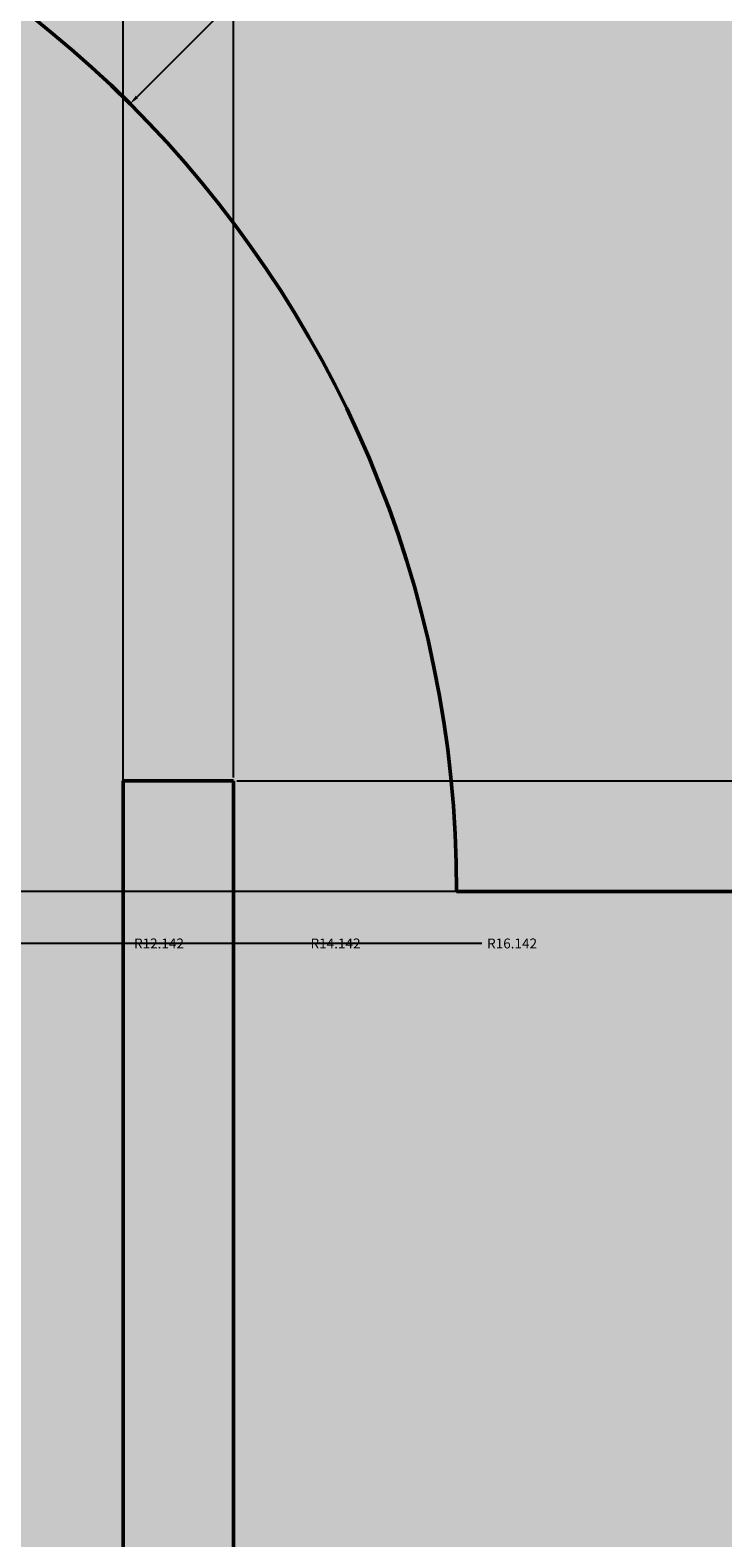
# Model space of a CAD drawing. Units: inches. Extents: x -12 to 334, y -10 to 186.
# Tile 55 of 77: x 244 to 257, y 69 to 96. Entities that reach past the tile are written whole.
import ezdxf

# ---------------------------------------------------------------- set-up
doc = ezdxf.new("R2010")
doc.units = ezdxf.units.IN
doc.header["$MEASUREMENT"] = 0
for name, color, linetype, lineweight in [('M-DIMS', 2, 'Continuous', 18), ('M-EQPM', 7, 'Continuous', 50), ('M-EQPM-PATT', 8, 'Continuous', 18)]:
    doc.layers.add(name, color=color, linetype=linetype, lineweight=lineweight)
doc.styles.get("Standard").update_dxf_attribs({"font": 'arial.ttf'})
doc.dimstyles.get("Standard").update_dxf_attribs({"dimtxt": 0.18, "dimasz": 0.18, "dimexe": 0.18, "dimexo": 0.0625, "dimgap": 0.09, "dimtad": 0, "dimtih": 1, "dimtoh": 1, "dimdec": 4, "dimzin": 0, "dimdsep": 46, "dimtxsty": 'Standard', "dimcen": 0.09, "dimadec": 0, "dimazin": 0, "dimtfac": 1, "dimtdec": 4, "dimtofl": 0, "dimtmove": 0, "dimatfit": 3, "dimfxl": 1, "dimtolj": 1, "dimtzin": 0, "dimarcsym": 0})

# ---------------------------------------------------------------- blocks, each defined once
blk = doc.blocks.new('*D1')
at = {"layer": 'Defpoints', "color": 0, "transparency": 16777216}
for p in [(281.426, 91.899), (3.376, 80.692), (281.426, 14.304)]:
    blk.add_point(p, dxfattribs=at)
at = {"layer": 'M-DIMS', "color": 0, "lineweight": -2, "transparency": 16777216}
for p, q in [((281.426, 91.836), (281.426, 14.124)), ((3.376, 80.629), (3.376, 14.124)), ((3.556, 14.304), (141.935, 14.304)), ((281.246, 14.304), (142.867, 14.304))]:
    blk.add_line(p, q, dxfattribs=at)
at = {"layer": 'M-DIMS', "color": 0, "transparency": 16777216}
for points in [[(3.556, 14.334), (3.556, 14.274), (3.376, 14.304)], [(281.246, 14.334), (281.246, 14.274), (281.426, 14.304)]]:
    blk.add_solid(points, dxfattribs=at)
at = {"layer": 'M-DIMS', "color": 0, "transparency": 16777216, "insert": (142.401, 14.304), "char_height": 0.18, "attachment_point": 5}
blk.add_mtext('\\A1;278.05', dxfattribs=at)
blk = doc.blocks.new('*D17')
at = {"layer": 'Defpoints', "color": 0, "transparency": 16777216}
for p in [(106.177, 102.896), (105.892, 56.321), (295.976, 56.321)]:
    blk.add_point(p, dxfattribs=at)
at = {"layer": 'M-DIMS', "color": 0, "lineweight": -2, "transparency": 16777216}
for p, q in [((106.24, 102.896), (296.156, 102.896)), ((295.976, 102.716), (295.976, 79.79)), ((295.976, 56.501), (295.976, 79.426)), ((105.954, 56.321), (296.156, 56.321))]:
    blk.add_line(p, q, dxfattribs=at)
at = {"layer": 'M-DIMS', "color": 0, "transparency": 16777216}
for points in [[(295.946, 102.716), (296.006, 102.716), (295.976, 102.896)], [(295.946, 56.501), (296.006, 56.501), (295.976, 56.321)]]:
    blk.add_solid(points, dxfattribs=at)
at = {"layer": 'M-DIMS', "color": 0, "transparency": 16777216, "insert": (295.976, 79.608), "char_height": 0.18, "attachment_point": 5}
blk.add_mtext('\\A1;46.575', dxfattribs=at)
blk = doc.blocks.new('*D36')
at = {"layer": 'Defpoints', "color": 0, "transparency": 16777216}
for p in [(247.935, 169.385), (245.935, 82.697), (247.935, 82.697)]:
    blk.add_point(p, dxfattribs=at)
at = {"layer": 'M-DIMS', "color": 0, "lineweight": -2, "transparency": 16777216}
for p, q in [((245.935, 82.759), (245.935, 169.565)), ((246.115, 169.385), (246.786, 169.385)), ((247.755, 169.385), (247.085, 169.385)), ((247.935, 82.759), (247.935, 169.565))]:
    blk.add_line(p, q, dxfattribs=at)
at = {"layer": 'M-DIMS', "color": 0, "transparency": 16777216}
for points in [[(246.115, 169.415), (246.115, 169.355), (245.935, 169.385)], [(247.755, 169.415), (247.755, 169.355), (247.935, 169.385)]]:
    blk.add_solid(points, dxfattribs=at)
at = {"layer": 'M-DIMS', "color": 0, "transparency": 16777216, "insert": (246.935, 169.385), "char_height": 0.18, "attachment_point": 5}
blk.add_mtext('\\A1;2', dxfattribs=at)
blk = doc.blocks.new('*D37')
at = {"layer": 'Defpoints', "color": 0, "transparency": 16777216}
for p in [(245.935, 169.385), (232.576, 46.854), (245.935, 46.854)]:
    blk.add_point(p, dxfattribs=at)
at = {"layer": 'M-DIMS', "color": 0, "lineweight": -2, "transparency": 16777216}
for p, q in [((232.576, 46.917), (232.576, 169.565)), ((232.756, 169.385), (238.871, 169.385)), ((245.755, 169.385), (239.641, 169.385)), ((245.935, 46.917), (245.935, 169.565))]:
    blk.add_line(p, q, dxfattribs=at)
at = {"layer": 'M-DIMS', "color": 0, "transparency": 16777216}
for points in [[(232.756, 169.415), (232.756, 169.355), (232.576, 169.385)], [(245.755, 169.415), (245.755, 169.355), (245.935, 169.385)]]:
    blk.add_solid(points, dxfattribs=at)
at = {"layer": 'M-DIMS', "color": 0, "transparency": 16777216, "insert": (239.256, 169.385), "char_height": 0.18, "attachment_point": 5}
blk.add_mtext('\\A1;13.36', dxfattribs=at)
blk = doc.blocks.new('*D38')
at = {"layer": 'Defpoints', "color": 0, "transparency": 16777216}
for p in [(247.935, 82.697), (247.935, 46.854), (295.976, 46.854)]:
    blk.add_point(p, dxfattribs=at)
at = {"layer": 'M-DIMS', "color": 0, "lineweight": -2, "transparency": 16777216}
for p, q in [((247.998, 82.697), (296.156, 82.697)), ((295.976, 82.517), (295.976, 64.957)), ((295.976, 47.034), (295.976, 64.594)), ((247.998, 46.854), (296.156, 46.854))]:
    blk.add_line(p, q, dxfattribs=at)
at = {"layer": 'M-DIMS', "color": 0, "transparency": 16777216}
for points in [[(295.946, 82.517), (296.006, 82.517), (295.976, 82.697)], [(295.946, 47.034), (296.006, 47.034), (295.976, 46.854)]]:
    blk.add_solid(points, dxfattribs=at)
at = {"layer": 'M-DIMS', "color": 0, "transparency": 16777216, "insert": (295.976, 64.775), "char_height": 0.18, "attachment_point": 5}
blk.add_mtext('\\A1;35.84', dxfattribs=at)
blk = doc.blocks.new('*D39')
at = {"layer": 'Defpoints', "color": 0, "transparency": 16777216}
for p in [(279.726, 80.692), (-11.174, 45.854), (269.381, 45.854)]:
    blk.add_point(p, dxfattribs=at)
at = {"layer": 'M-DIMS', "color": 0, "lineweight": -2, "transparency": 16777216}
for p, q in [((279.664, 80.692), (-11.354, 80.692)), ((-11.174, 80.512), (-11.174, 63.455)), ((-11.174, 46.034), (-11.174, 63.091)), ((269.318, 45.854), (-11.354, 45.854))]:
    blk.add_line(p, q, dxfattribs=at)
at = {"layer": 'M-DIMS', "color": 0, "transparency": 16777216}
for points in [[(-11.204, 80.512), (-11.144, 80.512), (-11.174, 80.692)], [(-11.204, 46.034), (-11.144, 46.034), (-11.174, 45.854)]]:
    blk.add_solid(points, dxfattribs=at)
at = {"layer": 'M-DIMS', "color": 0, "transparency": 16777216, "insert": (-11.174, 63.273), "char_height": 0.18, "attachment_point": 5}
blk.add_mtext('\\A1;34.84', dxfattribs=at)
blk = doc.blocks.new('*D40')
at = {"layer": 'Defpoints', "color": 0, "transparency": 16777216}
for p in [(278.229, 116.208), (187.394, 91.899)]:
    blk.add_point(p, dxfattribs=at)
at = {"layer": 'M-DIMS', "color": 0, "lineweight": -2, "transparency": 16777216}
for p, q in [((332.73, 130.793), (278.403, 116.254)), ((187.394, 91.809), (187.394, 91.989)), ((187.304, 91.899), (187.484, 91.899))]:
    blk.add_line(p, q, dxfattribs=at)
at = {"layer": 'M-DIMS', "color": 0, "transparency": 16777216}
blk.add_solid([(278.395, 116.283), (278.411, 116.225), (278.229, 116.208)], dxfattribs=at)
at = {"layer": 'M-DIMS', "color": 0, "transparency": 16777216, "insert": (333.21, 130.793), "char_height": 0.18, "attachment_point": 5}
blk.add_mtext('\\A1;R94.03', dxfattribs=at)
blk = doc.blocks.new('*D41')
at = {"layer": 'Defpoints', "color": 0, "transparency": 16777216}
for p in [(190.169, 91.899), (277.343, 68.515)]:
    blk.add_point(p, dxfattribs=at)
at = {"layer": 'M-DIMS', "color": 0, "lineweight": -2, "transparency": 16777216}
for p, q in [((190.169, 91.809), (190.169, 91.989)), ((190.079, 91.899), (190.259, 91.899)), ((329.648, 54.485), (277.517, 68.469)), ((329.828, 54.485), (329.648, 54.485))]:
    blk.add_line(p, q, dxfattribs=at)
at = {"layer": 'M-DIMS', "color": 0, "transparency": 16777216}
blk.add_solid([(277.525, 68.498), (277.509, 68.44), (277.343, 68.515)], dxfattribs=at)
at = {"layer": 'M-DIMS', "color": 0, "transparency": 16777216, "insert": (330.307, 54.485), "char_height": 0.18, "attachment_point": 5}
blk.add_mtext('\\A1;R90.26', dxfattribs=at)
blk = doc.blocks.new('*D43')
at = {"layer": 'Defpoints', "color": 0, "transparency": 16777216}
for p in [(246.06, 94.98), (231.776, 80.692)]:
    blk.add_point(p, dxfattribs=at)
at = {"layer": 'M-DIMS', "color": 0, "lineweight": -2, "transparency": 16777216}
for p, q in [((254.631, 103.553), (246.187, 95.108)), ((254.811, 103.553), (254.631, 103.553)), ((231.686, 80.692), (231.866, 80.692)), ((231.776, 80.602), (231.776, 80.782))]:
    blk.add_line(p, q, dxfattribs=at)
at = {"layer": 'M-DIMS', "color": 0, "transparency": 16777216}
blk.add_solid([(246.166, 95.129), (246.209, 95.086), (246.06, 94.98)], dxfattribs=at)
at = {"layer": 'M-DIMS', "color": 0, "transparency": 16777216, "insert": (255.36, 103.553), "char_height": 0.18, "attachment_point": 5}
blk.add_mtext('\\A1;R20.204', dxfattribs=at)
blk = doc.blocks.new('*D45')
at = {"layer": 'Defpoints', "color": 0, "transparency": 16777216}
for p in [(226.608, 79.754), (242.751, 79.75)]:
    blk.add_point(p, dxfattribs=at)
at = {"layer": 'M-DIMS', "color": 0, "lineweight": -2, "transparency": 16777216}
for p, q in [((226.518, 79.754), (226.698, 79.754)), ((226.608, 79.664), (226.608, 79.844)), ((252.436, 79.748), (242.931, 79.75))]:
    blk.add_line(p, q, dxfattribs=at)
at = {"layer": 'M-DIMS', "color": 0, "transparency": 16777216}
blk.add_solid([(242.931, 79.78), (242.931, 79.72), (242.751, 79.75)], dxfattribs=at)
at = {"layer": 'M-DIMS', "color": 0, "transparency": 16777216, "insert": (252.985, 79.748), "char_height": 0.18, "attachment_point": 5}
blk.add_mtext('\\A1;R16.142', dxfattribs=at)
blk = doc.blocks.new('*D46')
at = {"layer": 'Defpoints', "color": 0, "transparency": 16777216}
for p in [(226.608, 79.754), (240.751, 79.75)]:
    blk.add_point(p, dxfattribs=at)
at = {"layer": 'M-DIMS', "color": 0, "lineweight": -2, "transparency": 16777216}
for p, q in [((226.518, 79.754), (226.698, 79.754)), ((226.608, 79.664), (226.608, 79.844)), ((249.236, 79.748), (240.931, 79.75))]:
    blk.add_line(p, q, dxfattribs=at)
at = {"layer": 'M-DIMS', "color": 0, "transparency": 16777216}
blk.add_solid([(240.931, 79.78), (240.931, 79.72), (240.751, 79.75)], dxfattribs=at)
at = {"layer": 'M-DIMS', "color": 0, "transparency": 16777216, "insert": (249.785, 79.748), "char_height": 0.18, "attachment_point": 5}
blk.add_mtext('\\A1;R14.142', dxfattribs=at)
blk = doc.blocks.new('*D47')
at = {"layer": 'Defpoints', "color": 0, "transparency": 16777216}
for p in [(226.608, 79.754), (238.751, 79.75)]:
    blk.add_point(p, dxfattribs=at)
at = {"layer": 'M-DIMS', "color": 0, "lineweight": -2, "transparency": 16777216}
for p, q in [((226.518, 79.754), (226.698, 79.754)), ((226.608, 79.664), (226.608, 79.844)), ((246.036, 79.748), (238.931, 79.75))]:
    blk.add_line(p, q, dxfattribs=at)
at = {"layer": 'M-DIMS', "color": 0, "transparency": 16777216}
blk.add_solid([(238.931, 79.78), (238.931, 79.72), (238.751, 79.75)], dxfattribs=at)
at = {"layer": 'M-DIMS', "color": 0, "transparency": 16777216, "insert": (246.585, 79.748), "char_height": 0.18, "attachment_point": 5}
blk.add_mtext('\\A1;R12.142', dxfattribs=at)

msp = doc.modelspace()

# ---------------------------------------------------------------- hatches: boundary and pattern name
at = {"layer": 'M-EQPM-PATT', "transparency": 33554556}
h = msp.add_hatch(color=256, dxfattribs=at)
h.set_gradient(color1=(248, 206, 179), color2=(248, 206, 179), tint=1)
h.paths.add_polyline_path([(179.7818, 136.8871), (126.9567, 136.8871), (106.1771, 100.8958), (171.5458, 100.8958)])
h.paths.add_polyline_path([(268.3808, 136.9435), (214.0166, 136.9435), (214.0166, 154.8345), (196.3421, 154.8345), (196.3421, 136.8871), (179.7818, 136.8871), (171.5458, 100.8958), (231.7758, 100.8958, -0.4142136), (251.9801, 80.6915), (279.7263, 80.6915, 0.1631825)])
at = {"layer": 'M-EQPM-PATT'}
h = msp.add_hatch(color=256, dxfattribs=at)
h.set_gradient(color1=(94, 103, 175), color2=(94, 103, 175), tint=1)
h.paths.add_polyline_path([(129.093, 89.8963), (86.8879, 89.8963), (86.8879, 69.6117), (129.093, 69.6117)], flags=17)
h.paths.add_polyline_path([(170.9079, 89.8963), (130.8573, 89.8963), (130.8573, 69.6117), (170.9079, 69.6117)], flags=17)
h.paths.add_polyline_path([(216.4278, 89.8963), (172.6722, 89.8963), (172.6722, 69.6117), (216.4278, 69.6117)], flags=17)
h.paths.add_polyline_path([(245.9354, 82.6969), (247.9354, 82.6969), (247.9354, 46.8541), (268.3808, 46.8541, 0.0998398), (279.7263, 80.6915), (251.9801, 80.6915, 0.4142136), (231.7758, 100.8958), (84.7229, 100.8958), (84.7229, 109.0583), (83.7229, 109.0583), (83.7229, 95.8963), (129.093, 95.8963), (129.093, 98.1081), (130.8573, 98.1081), (130.8573, 95.8963), (170.9079, 95.8963), (170.9079, 98.1081), (172.6722, 98.1081), (172.6722, 95.8963), (216.4278, 95.8963), (216.4278, 98.1081), (218.1922, 98.1081), (218.1922, 95.8963), (226.6083, 95.8963, -1), (226.6083, 63.6117), (218.1922, 63.6117), (218.1922, 61.1045), (216.4278, 61.1045), (216.4278, 63.6117), (172.6722, 63.6117), (172.6722, 61.1045), (170.9079, 61.1045), (170.9079, 63.6117), (130.8573, 63.6117), (130.8573, 61.1045), (129.093, 61.1045), (129.093, 63.6117), (87.8879, 63.6117), (87.8879, 56.3205), (105.8919, 56.3205), (105.8919, 28.8541), (115.8919, 28.8541), (115.8919, 46.8541), (222.5761, 46.8541), (222.5761, 30.8541), (232.5761, 30.8541), (232.5761, 46.8541), (245.9354, 46.8541)])
h.paths.add_polyline_path([(86.8879, 89.8963), (75.9244, 89.8963), (75.9244, 69.6117), (86.8879, 69.6117)])
h.paths.add_polyline_path([(83.7229, 109.0583), (75.9244, 109.0583), (75.9244, 95.8963), (83.7229, 95.8963)])
h.paths.add_polyline_path([(226.6083, 89.8963), (218.1922, 89.8963), (218.1922, 69.6117), (226.6083, 69.6117, 1)], flags=17)
h = msp.add_hatch(color=256, dxfattribs=at)
h.set_gradient(color1=(0, 0, 255), color2=(0, 0, 255), tint=1)
h.paths.add_polyline_path([(84.7229, 100.8958), (84.7229, 109.0583), (83.7229, 109.0583), (83.7229, 95.8963), (129.093, 95.8963), (129.093, 98.1081), (130.8573, 98.1081), (130.8573, 95.8963), (170.9079, 95.8963), (170.9079, 98.1081), (172.6722, 98.1081), (172.6722, 95.8963), (216.4278, 95.8963), (216.4278, 98.1081), (218.1922, 98.1081), (218.1922, 95.8963), (226.6083, 95.8963, -1), (226.6083, 63.6117), (218.1922, 63.6117), (218.1922, 61.1045), (216.4278, 61.1045), (216.4278, 63.6117), (172.6722, 63.6117), (172.6722, 61.1045), (170.9079, 61.1045), (170.9079, 63.6117), (130.8573, 63.6117), (130.8573, 61.1045), (129.093, 61.1045), (129.093, 63.6117), (87.8879, 63.6117), (87.8879, 56.3205), (105.8919, 56.3205), (105.8919, 28.8541), (115.8919, 28.8541), (115.8919, 46.8541), (222.5761, 46.8541), (222.5761, 30.8541), (232.5761, 30.8541), (232.5761, 46.8541), (245.9354, 46.8541), (245.9354, 82.6969), (247.9354, 82.6969), (247.9354, 46.8541), (268.3808, 46.8541, 0.0998398), (279.7263, 80.6915), (251.9801, 80.6915, 0.4142136), (231.7758, 100.8958)])
h = msp.add_hatch(color=256, dxfattribs=at)
h.set_gradient(color1=(241, 235, 31), color2=(244, 238, 81), tint=1)
h.paths.add_polyline_path([(245.9354, 46.8541), (247.9354, 46.8541), (247.9354, 82.6969), (245.9354, 82.6969)])

# ---------------------------------------------------------------- linework, layer by layer
at = {"layer": 'M-EQPM'}
for p, q in [((245.9354, 82.6969), (245.9354, 46.8541)), ((245.9354, 82.6969), (247.9354, 82.6969)), ((247.9354, 82.6969), (247.9354, 46.8541)), ((251.9801, 80.6915), (279.7263, 80.6915))]:
    msp.add_line(p, q, dxfattribs=at)
msp.add_arc((231.7758, 80.6915), 20.2043, 0, 90, dxfattribs=at)

# ---------------------------------------------------------------- dimensions: what is measured, and where the dimension line sits
at = {"layer": 'M-DIMS'}
for base, p1, p2, override, picture, middle in [((245.9354, 169.3845), (232.5761, 46.8541), (245.9354, 46.8541), {"dimdec": 2, "dimlfac": 1, "dimrnd": 0, "dimzin": 0, "dimdsep": 46, "dimlunit": 2}, '*D37', (239.2558, 169.3845)), ((247.9354, 169.3845), (245.9354, 82.6969), (247.9354, 82.6969), {"dimdec": 0, "dimlfac": 1, "dimrnd": 0, "dimzin": 0, "dimdsep": 46, "dimlunit": 2}, '*D36', (246.9354, 169.3845)), ((281.4256, 14.3041), (3.3765, 80.6915), (281.4256, 91.8988), {"dimdec": 2, "dimlfac": 1, "dimrnd": 0, "dimzin": 0, "dimdsep": 46, "dimlunit": 2}, '*D1', (142.401, 14.3041))]:
    dim = msp.add_linear_dim(base=base, p1=p1, p2=p2, dimstyle='Standard', override=override, dxfattribs=at)
    dim.commit()
    dim.dimension.update_dxf_attribs({"geometry": picture, "text_midpoint": middle})
for center, mpoint, override, picture, middle in [((187.3936, 91.8988), (278.2291, 116.2078), {"dimdec": 2, "dimlfac": 1, "dimrnd": 0, "dimzin": 0, "dimdsep": 46, "dimlunit": 2}, '*D40', (332.7304, 130.7932)), ((231.7758, 80.6915), (246.0602, 94.9802), {"dimdec": 3, "dimlfac": 1, "dimrnd": 0, "dimzin": 0, "dimdsep": 46, "dimlunit": 2}, '*D43', (255.3603, 103.5535)), ((190.1689, 91.8988), (277.3431, 68.5153), {"dimdec": 2, "dimlfac": 1, "dimrnd": 0, "dimzin": 0, "dimdsep": 46, "dimlunit": 2}, '*D41', (330.3074, 54.4851)), ((226.6083, 79.754), (242.7506, 79.75), {"dimdec": 3, "dimlfac": 1, "dimrnd": 0, "dimzin": 0, "dimdsep": 46, "dimlunit": 2}, '*D45', (252.436, 79.7476)), ((226.6083, 79.754), (240.7506, 79.75), {"dimdec": 3, "dimlfac": 1, "dimrnd": 0, "dimzin": 0, "dimdsep": 46, "dimlunit": 2}, '*D46', (249.236, 79.7476)), ((226.6083, 79.754), (238.7506, 79.75), {"dimdec": 3, "dimlfac": 1, "dimrnd": 0, "dimzin": 0, "dimdsep": 46, "dimlunit": 2}, '*D47', (246.036, 79.7476))]:
    dim = msp.add_radius_dim(center=center, mpoint=mpoint, dimstyle='Standard', override=override, dxfattribs=at)
    dim.commit()
    dim.dimension.update_dxf_attribs({"geometry": picture, "text_midpoint": middle, "dimtype": 164})
for base, p1, p2, override, picture, middle in [((295.9756, 56.3205), (106.1771, 102.8958), (105.8919, 56.3205), {"dimdec": 3, "dimlfac": 1, "dimrnd": 0, "dimzin": 0, "dimdsep": 46, "dimlunit": 2}, '*D17', (295.9756, 79.6082)), ((295.9756, 46.8541), (247.9354, 82.6969), (247.9354, 46.8541), {"dimdec": 2, "dimlfac": 1, "dimrnd": 0, "dimzin": 0, "dimdsep": 46, "dimlunit": 2}, '*D38', (295.9756, 64.7755)), ((-11.1736, 45.8541), (279.7263, 80.6915), (269.3808, 45.8541), {"dimdec": 2, "dimlfac": 1, "dimrnd": 0, "dimzin": 0, "dimdsep": 46, "dimlunit": 2}, '*D39', (-11.1735, 63.2728))]:
    dim = msp.add_linear_dim(base=base, p1=p1, p2=p2, angle=90, dimstyle='Standard', override=override, dxfattribs=at)
    dim.commit()
    dim.dimension.update_dxf_attribs({"geometry": picture, "text_midpoint": middle})

doc.saveas('drawing.dxf')
